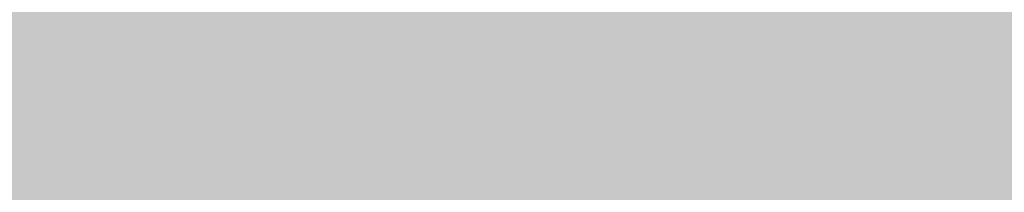
# Model space of a CAD drawing. Units: inches. Extents: x 2091 to 2899, y 967 to 2217.
# Tile 187 of 256: x 2203.16122 to 2203.18039, y 1152.25042 to 1152.25378. Entities that reach past the tile are written whole.
import ezdxf

# ---------------------------------------------------------------- set-up
doc = ezdxf.new("R2010")
doc.units = ezdxf.units.IN
doc.layers.add('A-WALL-PATT', color=141, linetype='Continuous', lineweight=13, true_color=0xadddf7)

msp = doc.modelspace()

# ---------------------------------------------------------------- hatches: boundary and pattern name
at = {"layer": 'A-WALL-PATT'}
h = msp.add_hatch(color=256, dxfattribs=at)
h.dxf.hatch_style = 1
h.paths.add_polyline_path([(2803.143603, 2050.919059), (2203.143603, 2050.919059), (2203.143603, 1090.919059), (2803.143603, 1090.919059)])
h.paths.add_polyline_path([(2635.79885, 1147.540465), (2674.524052, 1147.540465, 0.376086), (2678.529665, 1152.880202), (2678.529665, 1159.556473, 0.333335), (2674.524319, 1163.561846), (2674.524319, 1163.56185), (2674.524319, 1192.93439), (2635.805971, 1192.93439), (2597.087622, 1192.93439), (2597.087622, 1163.561846, 0.333335), (2593.082276, 1159.556473), (2593.082276, 1152.880202, 0.376086), (2597.087889, 1147.540465)], flags=0)
h.paths.add_polyline_path([(2436.010433, 1278.240778, 0.000483), (2435.952643, 1278.215027, -0.001328), (2435.935625, 1278.111693, -0.001711), (2436.11644, 1278.040758, 0.002185)], flags=0)
h.paths.add_polyline_path([(2794.143603, 1143.419059), (2794.143603, 1347.419059), (2543.370171, 1347.419059), (2543.370171, 1351.919059), (2794.143603, 1351.919059), (2794.143603, 1392.713555), (2793.947398, 1392.713555), (2793.947398, 1473.5369), (2794.143603, 1473.5369), (2794.143603, 1531.919059), (2650.143603, 1531.919059), (2650.143603, 1536.419059), (2794.143603, 1536.419059), (2794.143603, 1692.419059), (2609.375609, 1692.419059), (2609.375609, 1644.419059), (2604.875609, 1644.419059), (2604.875609, 1744.919059), (2609.375609, 1744.919059), (2609.375609, 1696.919059), (2794.143603, 1696.919059), (2794.143603, 1780.919059), (2609.643603, 1780.919059), (2493.875609, 1780.919059), (2493.875609, 1785.419059), (2609.643603, 1785.419059), (2794.143603, 1785.419059), (2794.143603, 1847.938821), (2793.951222, 1847.938821), (2793.951222, 1928.762166), (2794.143603, 1928.762166), (2794.143603, 1941.419059), (2614.143603, 1941.419059), (2614.143603, 1821.419059), (2609.643603, 1821.419059), (2609.643603, 1941.419059), (2392.143603, 1941.419059), (2392.143603, 1819.919059), (2387.643603, 1819.919059), (2387.643603, 1941.419059), (2212.143603, 1941.419059), (2212.143603, 1783.919059), (2392.143603, 1783.919059), (2392.143603, 1780.919059), (2212.143603, 1780.919059), (2212.143603, 1629.419059), (2387.643603, 1629.419059), (2387.643603, 1744.919059), (2392.143603, 1744.919059), (2392.143603, 1627.919059), (2317.143603, 1627.919059), (2317.143603, 1551.419059), (2317.143603, 1536.419059), (2459.383591, 1536.419059), (2459.383591, 1602.39648), (2463.883591, 1602.39648), (2463.883591, 1531.919059), (2456.643603, 1531.919059), (2456.643603, 1529.919059), (2452.143603, 1529.919059), (2452.143603, 1531.919059), (2312.643603, 1531.919059), (2312.643603, 1551.419059), (2306.143603, 1551.419059), (2306.143603, 1555.919059), (2308.143603, 1555.919059), (2308.143603, 1551.419059), (2312.643603, 1551.419059), (2312.643603, 1627.919059), (2212.143603, 1627.919059), (2212.143603, 1555.919059), (2270.143603, 1555.919059), (2270.143603, 1551.419059), (2212.143603, 1551.419059), (2212.143603, 1351.919059), (2272.143603, 1351.919059), (2272.143603, 1347.419059), (2212.143603, 1347.419059), (2212.143603, 1275.419059), (2308.143603, 1275.419059), (2308.143603, 1351.919059), (2452.143603, 1351.919059), (2452.143603, 1493.919059), (2456.643603, 1493.919059), (2456.643603, 1347.419059), (2312.643603, 1347.419059), (2312.643603, 1270.919059), (2212.143603, 1270.919059), (2212.143603, 1099.919059), (2281.237523, 1099.919059), (2282.871041, 1110.913803), (2282.008341, 1116.996603), (2278.557741, 1121.420403), (2268.205641, 1128.056203), (2272.087641, 1128.056203), (2273.812941, 1131.927003), (2279.420341, 1134.691903), (2285.027841, 1135.244903), (2287.615841, 1137.456803), (2288.047141, 1138.009803), (2289.341141, 1140.774703), (2291.066541, 1139.668703), (2292.360541, 1135.244903), (2295.379841, 1136.903803), (2296.242541, 1135.797903), (2297.105241, 1133.033003), (2300.124641, 1138.009803), (2303.143941, 1138.009803), (2304.437941, 1135.797903), (2303.143941, 1133.586003), (2306.594641, 1134.691903), (2307.888741, 1133.033003), (2310.908041, 1135.244903), (2313.927441, 1134.138903), (2315.62686, 1132.427102), (2308.320041, 1117.549603), (2290.203841, 1109.807903), (2288.909841, 1103.172103), (2289.272309, 1099.919059), (2434.918227, 1099.919059), (2431.593227, 1124.788059), (2429.930227, 1169.553059), (2430.927185, 1240.519694), (2435.658926, 1238.186126), (2437.135227, 1196.554059), (2438.798227, 1143.973059), (2442.678227, 1111.998059), (2446.558227, 1099.919059), (2794.143603, 1099.919059), (2794.143603, 1138.919059), (2548.032447, 1138.919059), (2548.032447, 1143.419059), (2548.032447, 1148.819059), (2546.668457, 1148.031559), (2528.685692, 1179.178622, 0.256256), (2512.032447, 1148.819059), (2512.032447, 1143.419059), (2512.032447, 1138.919059), (2507.532447, 1138.919059), (2507.532447, 1143.419059), (2507.532447, 1148.819059, 0.256256), (2490.879202, 1179.178622), (2472.896437, 1148.031559), (2471.532447, 1148.819059), (2471.532447, 1143.419059), (2467.032447, 1143.419059), (2467.032447, 1269.945786, 0.039061), (2460.909987, 1273.580059), (2467.032447, 1273.580059), (2467.032447, 1286.325364, 0.014511), (2465.216194, 1286.761905), (2467.032447, 1287.052576), (2467.032447, 1323.419059), (2471.532447, 1323.419059), (2471.532447, 1148.819059), (2489.532447, 1179.995973), (2490.896437, 1179.208473), (2490.879202, 1179.178622, -0.256256), (2507.532447, 1148.819059), (2507.532447, 1143.419059), (2512.032447, 1143.419059), (2512.032447, 1148.819059, -0.256256), (2528.685692, 1179.178622), (2528.668457, 1179.208473), (2530.032447, 1179.995973), (2548.032447, 1148.819059), (2548.032447, 1143.419059)], flags=16)
h.paths.add_polyline_path([(2607.768546, 1200.945083), (2607.768546, 1265.030625), (2597.087622, 1281.052011), (2619.784585, 1281.052011), (2627.795278, 1337.12686), (2635.79885, 1337.12686), (2643.816663, 1337.12686), (2651.827356, 1281.052011), (2674.524319, 1281.052011), (2663.843395, 1265.030625), (2663.843395, 1200.945083), (2635.805971, 1200.945083)], flags=0)
edge = h.paths.add_edge_path(flags=0)
edge.add_ellipse((13303.896215, 1272.998725), major_axis=(-10595.31304, 0.000001), ratio=0.842303870086, start_angle=0.6282372191, end_angle=0.6465540999, ccw=False)
edge.add_ellipse((2711.70045, 1156.852678), major_axis=(2.219769, 0), ratio=0.84230387, start_angle=111.535244, end_angle=180.628237, ccw=False)
edge.add_ellipse((13303.156292, 1272.998725), major_axis=(-10593.026306, 0), ratio=0.842303869544, start_angle=0.5282714718, end_angle=0.6465540971, ccw=False)
edge.add_line((2710.764596, 1175.333295), (2710.129986, 1175.333295))
edge.add_ellipse((2710.129986, 1176.579775), major_axis=(1.479846, 0), ratio=0.84230387, start_angle=180, end_angle=270, ccw=False)
edge.add_line((2708.65014, 1176.579775), (2708.65014, 1200.782914))
edge.add_ellipse((2710.129986, 1200.782914), major_axis=(1.479846, 0), ratio=0.84230387, start_angle=90, end_angle=180, ccw=False)
edge.add_line((2710.129986, 1202.029394), (2710.465075, 1202.029394))
edge.add_ellipse((13303.156292, 1272.998725), major_axis=(-10593.026306, 0), ratio=0.842303869544, start_angle=-0.0902290886, end_angle=0.3838667788, ccw=False)
edge.add_ellipse((2710.129986, 1290.927031), major_axis=(-1.479846, 0), ratio=0.84230387, start_angle=0, end_angle=90, ccw=False)
edge.add_line((2708.65014, 1290.927031), (2708.65014, 1315.13017))
edge.add_ellipse((2710.129986, 1315.13017), major_axis=(-1.479846, 0), ratio=0.84230387, start_angle=-90, end_angle=0, ccw=False)
edge.add_line((2710.129986, 1316.37665), (2710.706314, 1316.37665))
edge.add_ellipse((3238.40172, 1296.289566), major_axis=(528.234, 0), ratio=0.8423038695, start_angle=176.34957241, end_angle=177.82004969, ccw=False)
edge.add_ellipse((2775.063043, 1071.450696), major_axis=(313.307761, 0), ratio=0.8423038695, start_angle=102.12596555, end_angle=103.78052899, ccw=False)
edge.add_ellipse((2775.063043, 1078.305698), major_axis=(-305.302891, 0), ratio=0.8423038695, start_angle=-79.790461, end_angle=-77.55537271, ccw=False)
edge.add_ellipse((2695.141767, 1541.975383), major_axis=(-250.960216, 0), ratio=0.8423038695, start_angle=99.25656601, end_angle=102.55493264)
edge.add_line((2741.410326, 1334.214255), (2747.132545, 1337.378477))
edge.add_ellipse((2747.538616, 1336.857478), major_axis=(-0.739923, 0), ratio=0.8423039, start_angle=270, end_angle=307.93313, ccw=False)
edge.add_ellipse((2747.538616, 1336.857478), major_axis=(-0.739923, 0), ratio=0.8423039, start_angle=232.06687, end_angle=270, ccw=False)
edge.add_line((2747.944687, 1337.378477), (2753.666906, 1334.214255))
edge.add_ellipse((2799.935466, 1541.975383), major_axis=(250.960216, 0), ratio=0.8423038695, start_angle=257.44506736, end_angle=260.74343399)
edge.add_ellipse((2720.014189, 1078.305698), major_axis=(305.302891, 0), ratio=0.8423038695, start_angle=77.55537271, end_angle=79.790461, ccw=False)
edge.add_ellipse((2720.014189, 1071.450696), major_axis=(-313.307761, 0), ratio=0.8423038695, start_angle=256.21947101, end_angle=257.87403445, ccw=False)
edge.add_ellipse((2256.675512, 1296.289566), major_axis=(-528.234, 0), ratio=0.8423038695, start_angle=182.17995031, end_angle=183.65042759, ccw=False)
edge.add_line((2784.370918, 1316.37665), (2784.947247, 1316.37665))
edge.add_ellipse((2784.947247, 1315.13017), major_axis=(1.479846, 0), ratio=0.84230387, start_angle=0, end_angle=90, ccw=False)
edge.add_line((2786.427093, 1315.13017), (2786.427093, 1290.927031))
edge.add_ellipse((2784.947247, 1290.927031), major_axis=(1.479846, 0), ratio=0.84230387, start_angle=270, end_angle=360, ccw=False)
edge.add_ellipse((-7808.07906, 1272.998725), major_axis=(10593.026306, 0), ratio=0.842303869544, start_angle=-0.3838667788, end_angle=0.0902290886, ccw=False)
edge.add_line((2784.612157, 1202.029394), (2784.947247, 1202.029394))
edge.add_ellipse((2784.947247, 1200.782914), major_axis=(1.479846, 0), ratio=0.84230387, start_angle=0, end_angle=90, ccw=False)
edge.add_line((2786.427093, 1200.782914), (2786.427093, 1176.579775))
edge.add_ellipse((2784.947247, 1176.579775), major_axis=(-1.479846, 0), ratio=0.84230387, start_angle=90, end_angle=180, ccw=False)
edge.add_line((2784.947247, 1175.333295), (2784.312636, 1175.333295))
edge.add_ellipse((-7808.07906, 1272.998725), major_axis=(10593.026306, 0), ratio=0.842303869544, start_angle=-0.6186431963, end_angle=-0.5282714718, ccw=False)
edge.add_ellipse((2783.376783, 1156.852678), major_axis=(-2.219769, 0), ratio=0.84230387, start_angle=179.371763, end_angle=248.464757, ccw=False)
edge.add_ellipse((-7808.818983, 1272.998725), major_axis=(-10595.31304, 0.000004), ratio=0.842303865762, start_angle=179.3534459226, end_angle=179.3717628034, ccw=False)
edge.add_ellipse((2780.297303, 1153.500793), major_axis=(-5.246426, 0), ratio=0.84230387, start_angle=90, end_angle=179.353446, ccw=False)
edge.add_line((2780.297303, 1149.081708), (2714.77993, 1149.081708))
edge.add_ellipse((2714.77993, 1153.500793), major_axis=(5.246426, 0), ratio=0.84230387, start_angle=180.646554, end_angle=270, ccw=False)
edge = h.paths.add_edge_path(flags=0)
edge.add_line((2718.187367, 1151.007833), (2718.187367, 1170.472364))
edge.add_ellipse((2721.14706, 1170.472364), major_axis=(-2.959692, 0), ratio=0.84230387, start_angle=-90, end_angle=0, ccw=False)
edge.add_line((2721.14706, 1172.965324), (2773.930173, 1172.965324))
edge.add_ellipse((2773.930173, 1170.472364), major_axis=(-2.959692, 0), ratio=0.84230387, start_angle=180, end_angle=270, ccw=False)
edge.add_line((2776.889865, 1170.472364), (2776.889865, 1151.007833))
edge.add_line((2776.889865, 1151.007833), (2718.187367, 1151.007833))
edge = h.paths.add_edge_path(flags=0)
edge.add_line((2718.187367, 1180.23415), (2718.187367, 1199.057834))
edge.add_ellipse((2747.538616, 1320.39864), major_axis=(147.017924, 0), ratio=0.8423038695, start_angle=256.40186531, end_angle=283.59813469)
edge.add_line((2776.889865, 1199.057834), (2776.889865, 1180.23415))
edge.add_ellipse((2747.538616, 1301.574956), major_axis=(147.017924, 0), ratio=0.8423038695, start_angle=256.40186531, end_angle=283.59813469, ccw=False)
edge = h.paths.add_edge_path(flags=0)
edge.add_ellipse((13303.156292, 1272.998725), major_axis=(-10591.54646, 0), ratio=0.842303869555, start_angle=0.0555943135, end_angle=0.3777641939, ccw=False)
edge.add_line((2711.616859, 1262.72171), (2715.667408, 1249.495396))
edge.add_ellipse((6413.891963, 1241.691919), major_axis=(-3698.236159, 0), ratio=0.84230386955, start_angle=-0.120897369, end_angle=0.364076349)
edge.add_line((2715.761038, 1218.192455), (2711.934307, 1203.167361))
edge = h.paths.add_edge_path(flags=0)
edge.add_line((2718.187367, 1251.074566), (2716.002485, 1267.450435))
edge.add_ellipse((2742.151175, 1202.18954), major_axis=(81.772585, 0), ratio=0.84230387, start_angle=94.27742096, end_angle=111.8349538, ccw=False)
edge.add_line((2737.009748, 1270.930626), (2758.067484, 1270.930626))
edge.add_ellipse((2752.926058, 1202.18954), major_axis=(81.772585, 0), ratio=0.84230387, start_angle=68.1650462, end_angle=85.72257904, ccw=False)
edge.add_line((2779.074747, 1267.450435), (2776.889865, 1251.074566))
edge.add_ellipse((2750.338059, 1187.885356), major_axis=(79.579664, 0), ratio=0.84230387, start_angle=67.20808512, end_angle=85.1299304)
edge.add_line((2756.034656, 1254.743656), (2739.042576, 1254.743656))
edge.add_ellipse((2744.739174, 1187.885356), major_axis=(79.579664, 0), ratio=0.84230387, start_angle=94.8700696, end_angle=112.79191488)
edge = h.paths.add_edge_path(flags=0)
edge.add_line((2783.142926, 1203.167361), (2779.316194, 1218.192455))
edge.add_ellipse((-918.81473, 1241.691919), major_axis=(3698.236159, 0), ratio=0.84230386955, start_angle=-0.364076349, end_angle=0.120897369)
edge.add_line((2779.409825, 1249.495396), (2783.460373, 1262.72171))
edge.add_ellipse((-7808.07906, 1272.998725), major_axis=(-10591.54646, 0), ratio=0.84230386954, start_angle=179.6222358061, end_angle=179.9444056865, ccw=False)
edge = h.paths.add_edge_path(flags=0)
edge.add_ellipse((2734.200892, 1286.69044), major_axis=(-0.356609, 6.340078), ratio=0.60383358, start_angle=89.0020143, end_angle=253.657408, ccw=False)
edge.add_line((2730.369001, 1286.541806), (2730.369001, 1301.35198))
edge.add_line((2730.369001, 1301.35198), (2735.913311, 1305.214803))
edge.add_ellipse((2736.384917, 1304.734561), major_axis=(0.739923, 0), ratio=0.8423039, start_angle=90, end_angle=134.480211, ccw=False)
edge.add_line((2736.384917, 1305.357801), (2738.032783, 1305.357801))
edge.add_line((2738.032783, 1305.357801), (2738.032783, 1307.707927))
edge.add_ellipse((2794.201642, 1307.707927), major_axis=(56.168859, 0), ratio=0.84230387, start_angle=150.5614304, end_angle=180, ccw=False)
edge.add_ellipse((2700.875591, 1307.707927), major_axis=(-56.168859, 0), ratio=0.84230387, start_angle=180, end_angle=209.4385696, ccw=False)
edge.add_line((2757.04445, 1307.707927), (2757.04445, 1305.357801))
edge.add_line((2757.04445, 1305.357801), (2758.692316, 1305.357801))
edge.add_ellipse((2758.692316, 1304.734561), major_axis=(-0.739923, 0), ratio=0.8423039, start_angle=225.519789, end_angle=270, ccw=False)
edge.add_line((2759.163922, 1305.214803), (2764.708231, 1301.35198))
edge.add_line((2764.708231, 1301.35198), (2764.708231, 1286.541806))
edge.add_ellipse((2760.87634, 1286.69044), major_axis=(0.356609, 6.340078), ratio=0.60383358, start_angle=106.342592, end_angle=270.9979857, ccw=False)
edge.add_line((2757.04445, 1285.79709), (2757.04445, 1307.707927))
edge.add_ellipse((2700.875591, 1307.707927), major_axis=(-56.168859, 0), ratio=0.84230387, start_angle=180, end_angle=209.4385696)
edge.add_ellipse((2794.201642, 1307.707927), major_axis=(56.168859, 0), ratio=0.84230387, start_angle=150.5614304, end_angle=180)
edge.add_line((2738.032783, 1307.707927), (2738.032783, 1285.79709))
h.paths.add_polyline_path([(2417.812273, 1104.449704), (2413.492273, 1102.529704), (2410.612273, 1103.969704), (2409.172273, 1106.369704), (2407.252273, 1107.329704), (2406.292273, 1109.729704), (2405.332273, 1114.049704), (2405.332273, 1117.889704), (2406.292273, 1120.129704), (2407.252273, 1119.809704), (2408.848322, 1118.327658), (2410.173945, 1119.42417), (2410.211273, 1120.405704), (2411.040731, 1121.419054), (2410.699273, 1119.858704), (2410.173945, 1119.42417), (2410.088452, 1117.176109), (2411.132836, 1116.206324), (2413.972273, 1119.329704), (2416.852273, 1120.769704), (2416.869721, 1120.798784), (2417.035071, 1119.405116), (2417.896213, 1118.143384), (2418.292273, 1118.369704), (2419.544447, 1120.039269), (2419.360915, 1118.387487), (2419.032108, 1119.356151), (2418.398939, 1118.511926), (2419.252273, 1114.529704), (2418.794091, 1107.198795)], flags=0)
h.paths.add_polyline_path([(2508.870171, 1347.419059), (2508.370171, 1347.419059), (2508.370171, 1351.919059), (2508.870171, 1351.919059)], flags=0)
h.paths.add_polyline_path([(2473.370171, 1347.419059), (2472.370171, 1347.419059), (2467.870171, 1347.419059), (2467.870171, 1455.419059), (2472.370171, 1455.419059), (2472.370171, 1352.419059), (2473.370171, 1352.419059)], flags=0)
h.paths.add_polyline_path([(2352.106244, 1217.446197), (2349.226244, 1218.886197), (2347.786244, 1221.286197), (2345.866244, 1222.246197), (2344.906244, 1224.646197), (2343.946244, 1228.966197), (2343.946244, 1232.806197), (2344.906244, 1235.046197), (2345.866244, 1234.726197), (2347.462293, 1233.244152), (2348.787916, 1234.340663), (2348.825244, 1235.322197), (2349.654702, 1236.335547), (2349.313244, 1234.775197), (2348.787916, 1234.340663), (2348.702423, 1232.092603), (2349.746807, 1231.122817), (2352.586244, 1234.246197), (2355.466244, 1235.686197), (2355.483692, 1235.715277), (2355.649043, 1234.321609), (2356.510185, 1233.059877), (2356.906244, 1233.286197), (2358.158418, 1234.955762), (2357.974887, 1233.30398), (2357.646079, 1234.272644), (2357.012911, 1233.428419), (2357.866244, 1229.446197), (2357.408062, 1222.115288), (2356.426244, 1219.366197)], flags=0)
h.paths.add_polyline_path([(2348.2968, 1112.22442), (2347.0138, 1112.31042), (2345.5298, 1114.12742), (2345.7318, 1115.85842), (2346.8118, 1116.98242), (2346.8118, 1114.64642), (2345.8668, 1114.21442), (2346.8798, 1114.30042)], flags=0)
h.paths.add_polyline_path([(2347.0138, 1110.92642), (2346.2718, 1110.49342), (2346.6098, 1111.18642)], flags=0)
h.paths.add_polyline_path([(2345.8668, 1118.19442), (2345.5298, 1117.32942), (2343.7078, 1118.02142), (2344.3828, 1118.62642)], flags=0)
h.paths.add_polyline_path([(2346.6768, 1109.28242), (2346.0698, 1108.07142), (2345.8668, 1110.06142)], flags=0)
h.paths.add_polyline_path([(2345.0568, 1119.75142), (2343.6398, 1119.75142), (2343.9778, 1121.13542)], flags=0)
h.paths.add_polyline_path([(2345.2598, 1116.55042), (2345.1248, 1115.85842), (2344.9218, 1115.68542), (2344.7198, 1116.37742)], flags=0)
h.paths.add_polyline_path([(2345.6648, 1112.31042), (2345.4618, 1111.53242), (2344.0448, 1111.96442), (2344.6518, 1112.57042)], flags=0)
h.paths.add_polyline_path([(2345.1918, 1113.34942), (2344.4498, 1113.86842), (2344.7198, 1114.38742)], flags=0)
h.paths.add_polyline_path([(2344.6518, 1116.80942), (2344.1798, 1115.68542), (2344.6518, 1115.33942), (2343.9098, 1114.90642), (2343.0328, 1115.94442), (2343.6398, 1116.46342)], flags=0)
h.paths.add_polyline_path([(2345.8668, 1106.68642), (2344.9898, 1105.56242), (2344.5168, 1106.60042)], flags=0)
h.paths.add_polyline_path([(2344.8548, 1110.06142), (2344.5168, 1109.28242), (2344.1128, 1109.71542)], flags=0)
h.paths.add_polyline_path([(2344.0448, 1113.52242), (2343.4378, 1113.08942), (2342.7628, 1113.95442)], flags=0)
h.paths.add_polyline_path([(2344.3148, 1111.01242), (2342.9648, 1110.32042), (2342.9648, 1111.09942)], flags=0)
h.paths.add_polyline_path([(2345.1248, 1104.69742), (2344.5848, 1103.74542), (2344.4498, 1104.26442)], flags=0)
h.paths.add_polyline_path([(2342.8298, 1121.22242), (2341.7498, 1120.53042), (2340.5358, 1121.04942), (2340.1308, 1121.82842), (2340.6708, 1122.95242), (2341.1428, 1121.82842), (2341.6148, 1122.00142)], flags=0)
h.paths.add_polyline_path([(2342.9648, 1119.75142), (2343.0328, 1118.45342), (2342.0878, 1118.02142), (2342.0198, 1119.49142)], flags=0)
h.paths.add_polyline_path([(2342.6948, 1116.89642), (2341.9528, 1116.63642), (2342.0198, 1117.32942)], flags=0)
h.paths.add_polyline_path([(2343.0328, 1112.22442), (2342.0198, 1111.79142), (2341.5478, 1112.22442), (2342.3578, 1113.34942)], flags=0)
h.paths.add_polyline_path([(2343.7748, 1104.43742), (2342.6278, 1102.88042), (2342.6948, 1104.61042), (2343.4378, 1105.12942)], flags=0)
h.paths.add_polyline_path([(2342.0198, 1115.07942), (2340.8058, 1115.51242), (2340.9408, 1116.37742)], flags=0)
h.paths.add_polyline_path([(2341.4808, 1120.09742), (2341.4808, 1119.40542), (2341.0758, 1119.57842), (2341.1428, 1120.09742)], flags=0)
h.paths.add_polyline_path([(2341.8178, 1114.47342), (2340.9408, 1113.08942), (2340.8058, 1114.56042)], flags=0)
h.paths.add_polyline_path([(2341.1428, 1118.54042), (2340.9408, 1116.98242), (2339.0508, 1117.67542), (2339.0508, 1118.62642)], flags=0)
h.paths.add_polyline_path([(2342.6948, 1101.66842), (2341.9528, 1101.84142), (2342.5598, 1102.36142)], flags=0)
h.paths.add_polyline_path([(2340.3328, 1119.66542), (2338.4438, 1119.57842), (2337.9038, 1120.35742), (2339.6578, 1120.61642)], flags=0)
h.paths.add_polyline_path([(2340.3328, 1115.33942), (2340.0628, 1113.69542), (2339.3878, 1115.33942)], flags=0)
h.paths.add_polyline_path([(2341.8178, 1103.83142), (2341.5478, 1102.88042), (2341.1428, 1103.65842)], flags=0)
h.paths.add_polyline_path([(2339.0508, 1122.86642), (2337.2958, 1121.82842), (2337.0938, 1123.12542), (2337.7688, 1123.81842)], flags=0)
h.paths.add_polyline_path([(2339.1178, 1121.74142), (2338.8478, 1121.22242), (2338.1738, 1121.04942), (2338.3758, 1121.56842)], flags=0)
h.paths.add_polyline_path([(2339.1858, 1119.31942), (2338.6458, 1118.71342), (2338.2408, 1118.10742), (2338.2408, 1118.88642)], flags=0)
h.paths.add_polyline_path([(2341.1428, 1101.92842), (2340.6028, 1101.23642), (2340.0628, 1101.84142), (2340.6028, 1102.36142)], flags=0)
h.paths.add_polyline_path([(2337.6338, 1117.76142), (2336.6208, 1118.28042), (2337.2958, 1118.97242)], flags=0)
h.paths.add_polyline_path([(2336.8238, 1119.57842), (2334.7988, 1118.97242), (2335.2038, 1120.35742), (2336.5538, 1120.87642)], flags=0)
h.paths.add_polyline_path([(2339.1178, 1100.45742), (2337.3638, 1100.54342), (2336.7558, 1101.23642)], flags=0)
h.paths.add_polyline_path([(2336.3508, 1122.43342), (2336.0138, 1121.91442), (2334.9338, 1122.43342), (2334.5288, 1123.47142), (2335.7438, 1122.77942)], flags=0)
h.paths.add_polyline_path([(2334.7318, 1120.87642), (2334.2588, 1120.35742), (2334.0568, 1120.78942), (2334.5968, 1121.30842)], flags=0)
h.paths.add_polyline_path([(2334.4618, 1122.17442), (2332.5718, 1121.30842), (2331.3568, 1122.17442), (2332.0998, 1122.86642)], flags=0)
h.paths.add_polyline_path([(2334.2588, 1118.54042), (2333.3818, 1118.45342), (2333.6518, 1119.31942)], flags=0)
h.paths.add_polyline_path([(2335.5418, 1102.27442), (2334.1918, 1102.62042), (2335.2718, 1103.31242)], flags=0)
h.paths.add_polyline_path([(2332.7068, 1119.66542), (2331.6948, 1120.44342), (2332.5048, 1120.78942)], flags=0)
h.paths.add_polyline_path([(2334.7318, 1101.14942), (2333.5168, 1101.58242), (2333.9888, 1101.75542)], flags=0)
h.paths.add_polyline_path([(2332.6398, 1116.63642), (2331.0868, 1116.29042), (2331.9648, 1118.19442)], flags=0)
h.paths.add_polyline_path([(2330.7498, 1121.56842), (2330.2768, 1120.27042), (2328.5228, 1119.31942), (2328.9948, 1121.04942)], flags=0)
h.paths.add_polyline_path([(2330.7498, 1118.62642), (2330.0078, 1117.50242), (2329.8728, 1118.02142)], flags=0)
h.paths.add_polyline_path([(2332.0998, 1102.36142), (2330.5468, 1102.01442), (2331.6948, 1102.96642)], flags=0)
h.paths.add_polyline_path([(2329.5348, 1113.60842), (2329.0628, 1112.31042), (2328.5898, 1113.34942)], flags=0)
h.paths.add_polyline_path([(2328.3878, 1117.84842), (2327.5098, 1116.55042), (2327.1728, 1117.76142)], flags=0)
h.paths.add_polyline_path([(2329.7378, 1106.51342), (2329.5348, 1105.30242), (2328.2528, 1106.08142)], flags=0)
h.paths.add_polyline_path([(2328.6578, 1114.38742), (2328.0498, 1114.12742), (2328.3198, 1114.90642)], flags=0)
h.paths.add_polyline_path([(2328.3198, 1112.22442), (2327.1058, 1112.13742), (2326.7008, 1112.65642)], flags=0)
h.paths.add_polyline_path([(2326.9028, 1115.25242), (2326.7008, 1114.12742), (2325.2158, 1113.60842), (2326.0928, 1115.33942)], flags=0)
h.paths.add_polyline_path([(2326.6328, 1108.33042), (2326.0928, 1107.37942), (2325.8908, 1108.50342), (2326.4978, 1109.10942)], flags=0)
h.paths.add_polyline_path([(2615.143603, 1531.919059), (2609.643603, 1531.919059), (2609.643603, 1620.419059), (2614.143603, 1620.419059), (2614.143603, 1536.419059), (2615.143603, 1536.419059)], flags=0)
h.paths.add_polyline_path([(2545.143603, 1563.419059), (2464.143603, 1563.419059), (2464.143603, 1632.419059), (2509.143603, 1632.419059), (2509.143603, 1627.919059), (2509.143603, 1603.919059), (2468.643603, 1603.919059), (2468.643603, 1567.919059), (2540.643603, 1567.919059), (2540.643603, 1591.919059), (2545.143603, 1591.919059)], flags=0)
h.paths.add_polyline_path([(2388.969048, 1549.985735), (2357.434181, 1549.985735), (2357.434181, 1623.360778), (2399.362777, 1623.360778), (2435.689465, 1623.360778), (2435.592547, 1602.559273), (2435.592547, 1602.39648), (2388.969048, 1602.39648)], flags=0)
h.paths.add_polyline_path([(2388.880628, 1555.809151), (2374.904429, 1555.809151), (2374.904429, 1600.571564), (2374.904429, 1615.457645), (2406.350877, 1615.457645), (2406.350877, 1618.939431), (2412.174293, 1615.457645), (2406.350877, 1611.97586), (2406.350877, 1615.457645), (2388.880628, 1615.457645)], flags=0)
h.paths.add_polyline_path([(2568.875609, 1644.419059), (2453.375609, 1644.419059), (2453.375609, 1785.419059), (2457.875609, 1785.419059), (2457.875609, 1648.919059), (2568.875609, 1648.919059)], flags=0)
h.paths.add_polyline_path([(2212.143603, 1945.919059), (2212.143603, 2041.919059), (2794.143603, 2041.919059), (2794.143603, 1945.919059)], flags=16)
h.paths.add_polyline_path([(2271.082728, 1964.317238), (2776.852968, 1964.317238), (2776.852968, 2037.169623), (2271.082728, 2037.169623)], flags=8)
h.paths.add_polyline_path([(2380.649285, 1536.824144), (2461.040809, 1536.824144), (2461.040809, 1554.652587), (2380.649285, 1554.652587)], flags=8)
h.paths.add_polyline_path([(2240.755709, 1609.725451), (2309.185829, 1609.725451), (2309.185829, 1617.698204), (2240.755709, 1617.698204)], flags=8)
h.paths.add_polyline_path([(2212.677255, 1313.504102), (2282.59152, 1313.504102), (2282.59152, 1322.745239), (2212.677255, 1322.745239)], flags=8)
h.paths.add_polyline_path([(2457.111976, 1114.778574), (2558.481581, 1114.778574), (2558.481581, 1142.219682), (2457.111976, 1142.219682)], flags=8)
h.paths.add_polyline_path([(2473.442337, 1273.010067), (2604.641226, 1273.010067), (2604.641226, 1318.346935), (2473.442337, 1318.346935)], flags=8)
h.paths.add_polyline_path([(2638.876302, 1626.977432), (2684.250367, 1627.976738), (2684.038483, 1637.597494), (2638.664417, 1636.598188)], flags=8)
h.paths.add_polyline_path([(2537.590554, 1453.793447), (2628.389547, 1453.793447), (2628.389547, 1475.344811), (2537.590554, 1475.344811)], flags=8)
h.paths.add_polyline_path([(2504.137638, 1714.632397), (2554.647187, 1714.632397), (2554.647187, 1730.237712), (2504.137638, 1730.237712)], flags=8)
h.paths.add_polyline_path([(2487.501181, 1575.651872), (2535.097121, 1575.651872), (2535.097121, 1598.377646), (2487.501181, 1598.377646)], flags=8)
h.paths.add_polyline_path([(2709.0994, 1735.710278), (2740.016601, 1735.710278), (2740.016601, 1749.937641), (2709.0994, 1749.937641)], flags=8)
h.paths.add_polyline_path([(2442.438424, 1792.171657), (2564.728835, 1792.171657), (2564.728835, 1842.000163), (2442.438424, 1842.000163)], flags=8)
h.paths.add_polyline_path([(2655.815801, 1809.644076), (2789.520142, 1806.693796), (2790.084977, 1832.291638), (2656.380635, 1835.241918)], flags=8)
h.paths.add_polyline_path([(2234.842697, 1797.720143), (2368.592851, 1794.768852), (2369.160718, 1820.504132), (2235.410564, 1823.455423)], flags=8)
h.paths.add_polyline_path([(2245.138466, 1644.006335), (2398.427733, 1640.6239), (2398.994842, 1666.32482), (2245.705575, 1669.707255)], flags=8)
h.paths.add_polyline_path([(2306.142847, 1431.168519), (2413.768314, 1428.793687), (2414.333148, 1454.391529), (2306.707682, 1456.76636)], flags=8)
h.paths.add_polyline_path([(2306.834582, 1458.233145), (2393.380484, 1456.323449), (2393.932808, 1481.354358), (2307.386907, 1483.264054)], flags=8)

doc.saveas('drawing.dxf')
